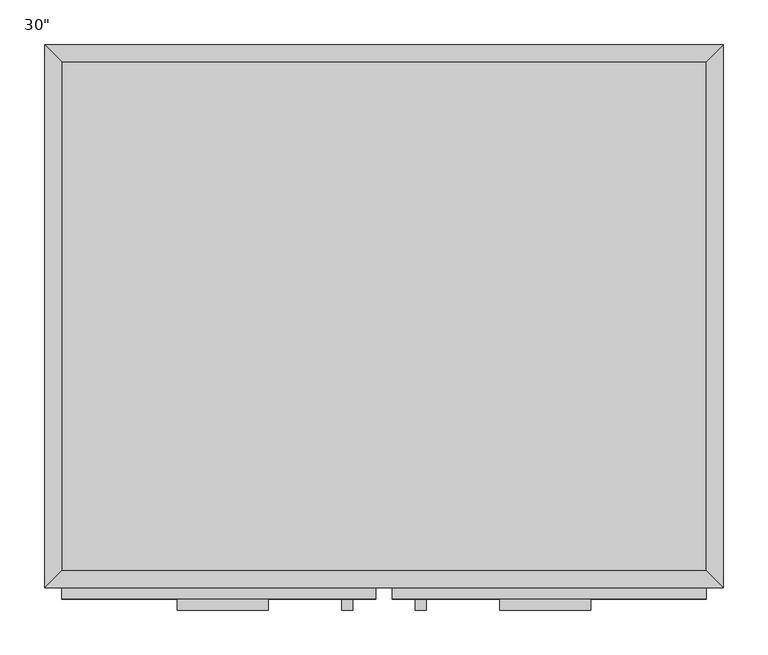
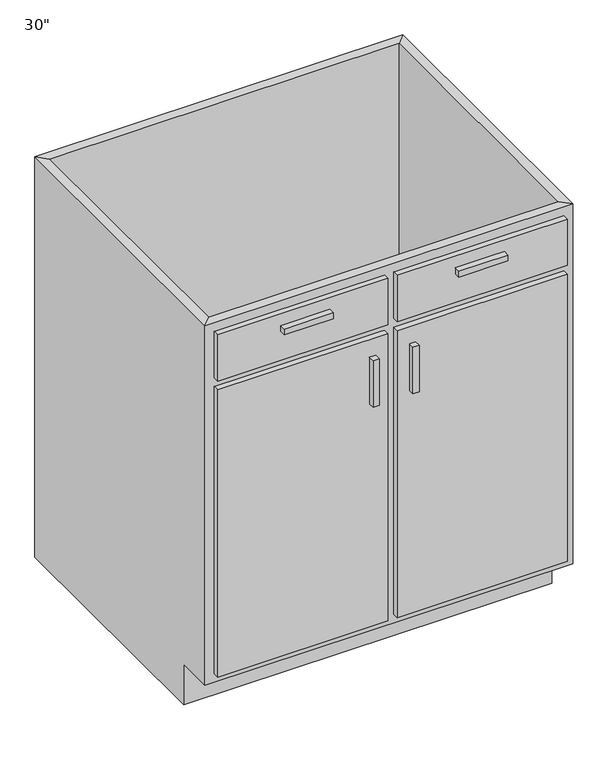
"""IFC4 building model written with IfcOpenShell, lengths in millimetres: furniture geometry."""

from ifc_helpers import new_model, si_unit, frame, origin, place, context, project, spatial, polyline, outline, extrude, faceted_brep, source, transform, mapped, element, save


def furniture_338da5bd(model_context):
    return source(origin(), model_context, "Body", "SolidModel", [
        faceted_brep([(380.6877049, -590.55, 876.3), (380.6877049, -590.55, 88.9), (-343.2122951, -590.55, 88.9), (-343.2122951, -590.55, 876.3), (-362.2622951, -609.6, 876.3), (399.7377049, -609.6, 876.3), (-362.2622951, -609.6, 88.9), (399.7377049, -609.6, 88.9), (-343.2122951, -533.4, 88.9), (-343.2122951, -19.05, 88.9), (-343.2122951, -19.05, 876.3), (-362.2622951, 0.0, 876.3), (-362.2622951, 0.0, 0.0), (-362.2622951, -533.4, 0.0), (-362.2622951, -533.4, 88.9), (380.6877049, -19.05, 88.9), (380.6877049, -19.05, 876.3), (399.7377049, 0.0, 876.3), (399.7377049, 0.0, 0.0), (380.6877049, -533.4, 88.9), (399.7377049, -533.4, 88.9), (399.7377049, -533.4, 0.0)], [[[0, 1, 2, 3]], [[0, 3, 4, 5]], [[5, 4, 6, 7]], [[2, 1, 7, 6]], [[3, 2, 8, 9, 10]], [[4, 3, 10, 11]], [[6, 4, 11, 12, 13, 14]], [[2, 6, 14, 8]], [[10, 9, 15, 16]], [[11, 10, 16, 17]], [[12, 11, 17, 18]], [[1, 0, 16, 15, 19]], [[0, 5, 17, 16]], [[5, 7, 20, 21, 18, 17]], [[7, 1, 19, 20]], [[8, 19, 15, 9]], [[18, 21, 13, 12]], [[13, 21, 20, 19, 8, 14]]]),
        extrude(outline(polyline([(-111.4372951, -635.0), (-213.0372951, -635.0), (-213.0372951, -622.3), (-111.4372951, -622.3), (-111.4372951, -635.0)])), frame((0.0, 0.0, 819.15), z_axis=(0.0, 0.0, 1.0), x_axis=(1.0, 0.0, 0.0)), (0.0, 0.0, 1.0), 12.7),
        extrude(outline(polyline([(250.5127049, -635.0), (148.9127049, -635.0), (148.9127049, -622.3), (250.5127049, -622.3), (250.5127049, -635.0)])), frame((0.0, 0.0, 819.15), z_axis=(0.0, 0.0, 1.0), x_axis=(1.0, 0.0, 0.0)), (0.0, 0.0, 1.0), 12.7),
        extrude(outline(polyline([(-16.1872951, -635.0), (-28.8872951, -635.0), (-28.8872951, -622.3), (-16.1872951, -622.3), (-16.1872951, -635.0)])), frame((0.0, 0.0, 596.9), z_axis=(0.0, 0.0, 1.0), x_axis=(1.0, 0.0, 0.0)), (0.0, 0.0, 1.0), 101.6),
        extrude(outline(polyline([(66.3627049, -635.0), (53.6627049, -635.0), (53.6627049, -622.3), (66.3627049, -622.3), (66.3627049, -635.0)])), frame((0.0, 0.0, 596.9), z_axis=(0.0, 0.0, 1.0), x_axis=(1.0, 0.0, 0.0)), (0.0, 0.0, 1.0), 101.6),
        extrude(outline(polyline([(380.6877049, -19.05), (380.6877049, -590.55), (-343.2122951, -590.55), (-343.2122951, -19.05), (380.6877049, -19.05)])), frame((0.0, 0.0, 88.9), z_axis=(0.0, 0.0, 1.0), x_axis=(1.0, 0.0, 0.0)), (0.0, 0.0, 1.0), 19.05),
        extrude(outline(polyline([(9.2127049, -622.3), (-343.2122951, -622.3), (-343.2122951, -609.6), (9.2127049, -609.6), (9.2127049, -622.3)])), frame((0.0, 0.0, 755.65), z_axis=(0.0, 0.0, 1.0), x_axis=(1.0, 0.0, 0.0)), (0.0, 0.0, 1.0), 101.6),
        extrude(outline(polyline([(380.6877049, -622.3), (28.2627049, -622.3), (28.2627049, -609.6), (380.6877049, -609.6), (380.6877049, -622.3)])), frame((0.0, 0.0, 755.65), z_axis=(0.0, 0.0, 1.0), x_axis=(1.0, 0.0, 0.0)), (0.0, 0.0, 1.0), 101.6),
        extrude(outline(polyline([(9.2127049, -622.3), (-343.2122951, -622.3), (-343.2122951, -609.6), (9.2127049, -609.6), (9.2127049, -622.3)])), frame((0.0, 0.0, 107.95), z_axis=(0.0, 0.0, 1.0), x_axis=(1.0, 0.0, 0.0)), (0.0, 0.0, 1.0), 628.65),
        extrude(outline(polyline([(380.6877049, -622.3), (28.2627049, -622.3), (28.2627049, -609.6), (380.6877049, -609.6), (380.6877049, -622.3)])), frame((0.0, 0.0, 107.95), z_axis=(0.0, 0.0, 1.0), x_axis=(1.0, 0.0, 0.0)), (0.0, 0.0, 1.0), 628.65),
    ])


if __name__ == "__main__":
    model = new_model("IFC4")
    model_context = context("Model", 3, world=origin())
    ifc_project = project(units=[si_unit("LENGTHUNIT", "METRE", prefix="MILLI")], contexts=[model_context])
    site = spatial("IfcSite", under=ifc_project)
    building = spatial("IfcBuilding", under=site)
    placement = place(None, origin())
    furniture_shape = furniture_338da5bd(model_context)
    element("IfcFurniture", 1, ObjectType="30\"", at=placement, inside=building, context=model_context, shape_type="MappedRepresentation", body=[
        mapped(furniture_shape, transform((0.0, 0.0, 0.0), x_axis=(1.0, 0.0, 0.0), y_axis=(0.0, 1.0, 0.0), z_axis=(0.0, 0.0, 1.0))),
    ])
    save(model, "model.ifc")

# Revit data of these elements
# Type "30\""
#   Assembly Code = "C1030410"
#   Depth = 2' - 0"
#   Height = 2' - 10 1/2"
#   Toe Depth = 0' - 3"
#   Toe Height = 0' - 3 1/2"
#   Width = 2' - 6"
#   Cabinet Material = none
#   Door/Drawer Material = none
#   Handle Material = Cabinets - Handles
#   Default Elevation = 0
# Element 1 (IfcFurniture, "30\"")
#   Materials on its faces: "Cabinets", "Cabinets - Handles"
# Materials
#   "Cabinets - Handles": class "Metal", colour RGB 57 57 57, transparency 0
#   "Cabinets": colour RGB 249 249 249, transparency 0
